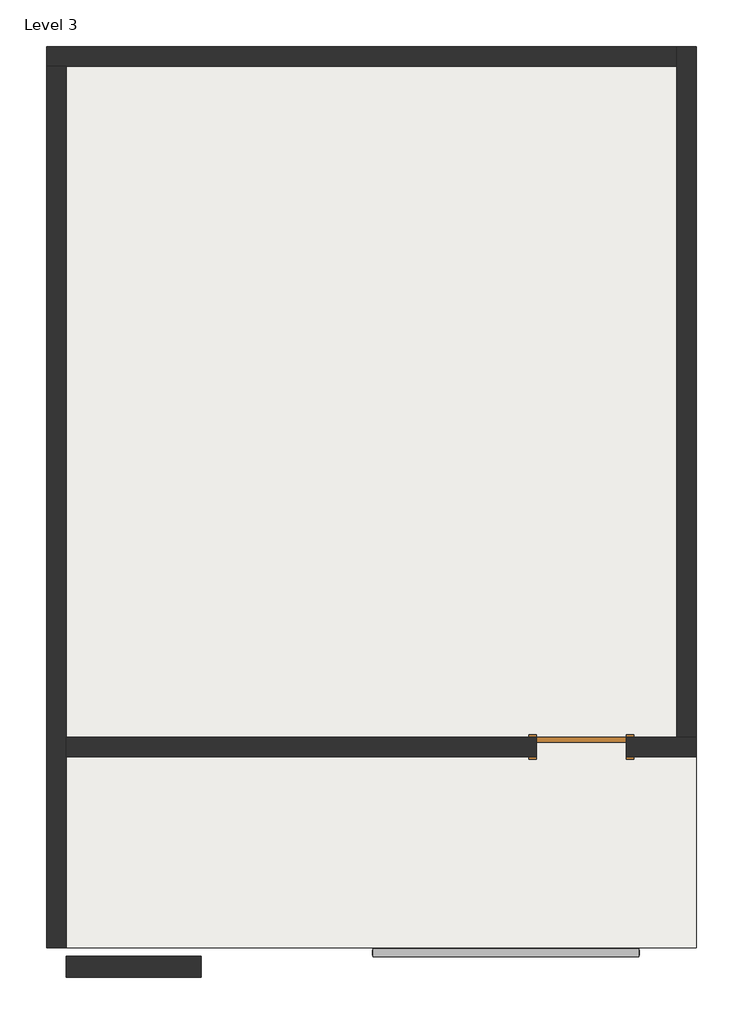
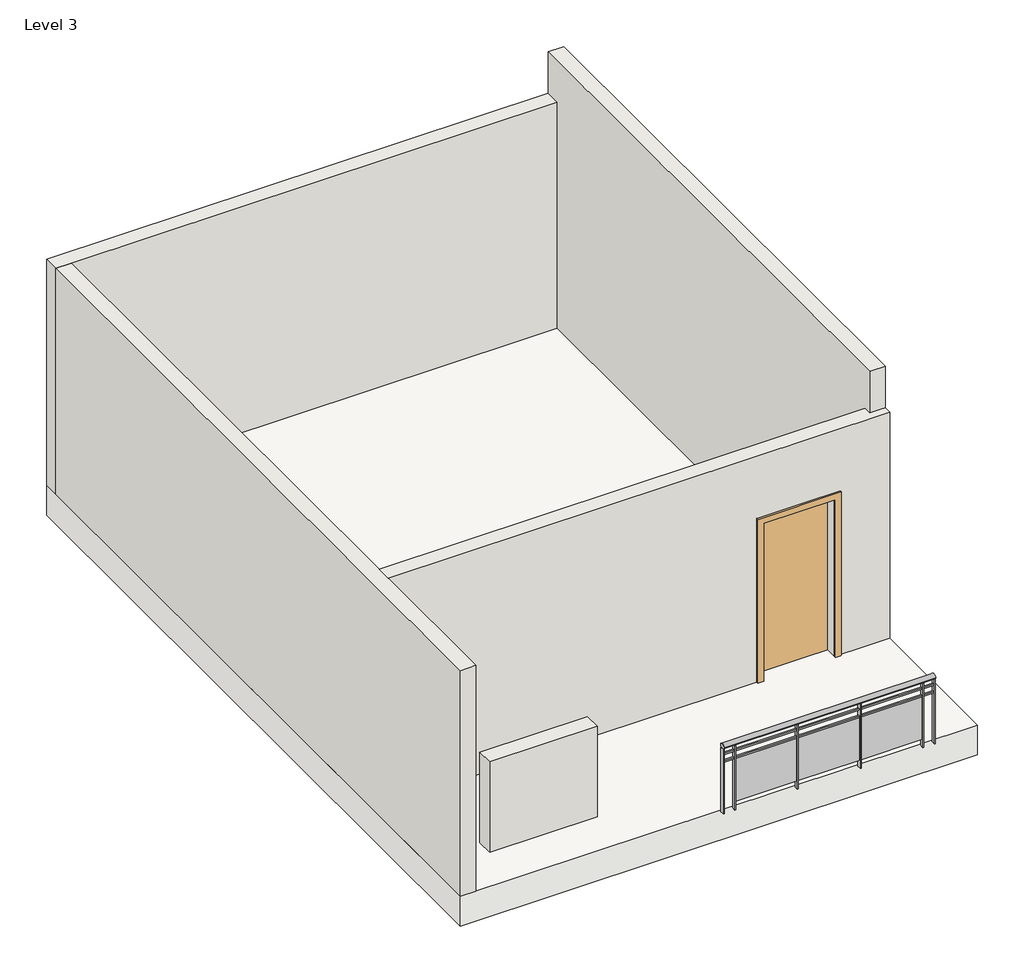
# One storey: 5 walls, 1 door, 1 railing, 1 slab.
"""IFC4 building model written with IfcOpenShell, lengths in millimetres."""

from ifc_helpers import new_model, si_unit, point, frame, origin, place, context, project, spatial, polyline, ellipse_curve, trimmed, outline, extrude, faceted_brep, transform, mapped, element, save
from ifc_brep_helpers import plane_surface, extruded_surface, advanced_brep
from components import m_single_flush_0915_x_2134mm_6a9e8738, walls_7_walls_7_d83e4491

model = new_model("IFC4")

# Units and contexts
model_context = context("Model", 3, world=origin())
ifc_project = project(units=[si_unit("LENGTHUNIT", "METRE", prefix="MILLI")], contexts=[model_context])

# Site, building, storey
site = spatial("IfcSite", under=ifc_project)
building = spatial("IfcBuilding", under=site)
storey = spatial("IfcBuildingStorey", under=building, Name="Level 3", Elevation=3048.0)

# Door
placement = place(None, origin())
m_single_flush_0915_x_2134mm_shape = m_single_flush_0915_x_2134mm_6a9e8738(model_context)
element("IfcDoor", 1, ObjectType="M_Single-Flush : 0915 x 2134mm", at=placement, inside=storey, context=model_context, shape_type="MappedRepresentation", body=[
    mapped(m_single_flush_0915_x_2134mm_shape, transform((-7079.0996792, -5453.0913939, 3048.0), x_axis=(1.0, 0.0, 0.0), y_axis=(0.0, 1.0, 0.0), z_axis=(0.0, 0.0, 1.0))),
])

# Railing
element("IfcRailing", 2, ObjectType="Glass Panel - Bottom Fill", at=placement, inside=storey, context=model_context, shape_type="SolidModel", body=[
    advanced_brep(
    [(-9197.0226654, -7500.5654668, 3948.0), (-9197.0226654, -7580.5654668, 3948.0), (-6496.1866069, -7500.5654668, 3948.0), (-6496.1866069, -7580.5654668, 3948.0)],
    [
        (0, 1, ellipse_curve(frame((-9197.0226654, -7540.5654668, 3948.0), z_axis=(-1.0, 0.0, 0.0), x_axis=(0.0, -1.0, 0.0)), 40.0, 30.0)),
        (1, 0, ellipse_curve(frame((-9197.0226654, -7540.5654668, 3948.0), z_axis=(-1.0, 0.0, 0.0), x_axis=(0.0, -1.0, 0.0)), 40.0, 30.0)),
        (2, 3, ellipse_curve(frame((-6496.1866069, -7540.5654668, 3948.0), z_axis=(1.0, 0.0, 0.0), x_axis=(0.0, -1.0, 0.0)), 40.0, 30.0)),
        (3, 2, ellipse_curve(frame((-6496.1866069, -7540.5654668, 3948.0), z_axis=(1.0, 0.0, 0.0), x_axis=(0.0, -1.0, 0.0)), 40.0, 30.0)),
        (1, 3),
        (2, 0),
    ],
    [
        plane_surface(frame((-9197.0226654, -7540.5654668, 3948.0), z_axis=(-1.0, 0.0, 0.0), x_axis=(0.0, 1.0, 0.0))),
        plane_surface(frame((-6496.1866069, -7540.5654668, 3948.0), z_axis=(1.0, 0.0, 0.0), x_axis=(0.0, 1.0, 0.0))),
        extruded_surface(trimmed(ellipse_curve(frame((-6496.1866069, -7540.5654668, 3948.0), z_axis=(-1.0, 0.0, 0.0), x_axis=(0.0, -1.0, 0.0)), 40.0, 30.0), [point((-6496.1866069, -7580.5654668, 3948.0))], [point((-6496.1866069, -7500.5654668, 3948.0))], True, "CARTESIAN"), (-2700.8360585, 0.0, 0.0), 2700.8360585),
        extruded_surface(trimmed(ellipse_curve(frame((-6496.1866069, -7540.5654668, 3948.0), z_axis=(-1.0, 0.0, 0.0), x_axis=(0.0, -1.0, 0.0)), 40.0, 30.0), [point((-6496.1866069, -7500.5654668, 3948.0))], [point((-6496.1866069, -7580.5654668, 3948.0))], True, "CARTESIAN"), (-2700.8360585, 0.0, 0.0), 2700.8360585),
    ],
    [
        (0, [[1, 2]]),
        (1, [[3, 4]]),
        (2, [[-2, 5, -3, 6]]),
        (3, [[-1, -6, -4, -5]]),
    ],
),
    extrude(outline(polyline([(-9197.0226654, -7549.9562319), (-9197.0226654, -7529.9562319), (-6496.1866069, -7529.9562319), (-6496.1866069, -7549.9562319), (-9197.0226654, -7549.9562319)])), frame((0.0, 0.0, 3828.0), z_axis=(0.0, 0.0, 1.0), x_axis=(1.0, 0.0, 0.0)), (0.0, 0.0, 1.0), 20.0),
    extrude(outline(polyline([(-9197.0226654, -7549.9562319), (-9197.0226654, -7529.9562319), (-6496.1866069, -7529.9562319), (-6496.1866069, -7549.9562319), (-9197.0226654, -7549.9562319)])), frame((0.0, 0.0, 3728.0), z_axis=(0.0, 0.0, 1.0), x_axis=(1.0, 0.0, 0.0)), (0.0, 0.0, 1.0), 20.0),
    extrude(outline(polyline([(-6652.6046361, -7514.9562319), (-6640.6046361, -7514.9562319), (-6640.6046361, -7564.9562319), (-6652.6046361, -7564.9562319), (-6652.6046361, -7514.9562319)])), frame((0.0, 0.0, 3048.0), z_axis=(0.0, 0.0, 1.0), x_axis=(1.0, 0.0, 0.0)), (0.0, 0.0, 1.0), 869.8465326),
    extrude(outline(polyline([(-7446.6046361, -7541.681042), (-6646.6046361, -7541.681042), (-6646.6046361, -7546.681042), (-7446.6046361, -7546.681042), (-7446.6046361, -7541.681042)])), frame((0.0, 0.0, 3148.0), z_axis=(0.0, 0.0, 1.0), x_axis=(1.0, 0.0, 0.0)), (0.0, 0.0, 1.0), 580.0),
    extrude(outline(polyline([(-7452.6046361, -7514.9562319), (-7440.6046361, -7514.9562319), (-7440.6046361, -7564.9562319), (-7452.6046361, -7564.9562319), (-7452.6046361, -7514.9562319)])), frame((0.0, 0.0, 3048.0), z_axis=(0.0, 0.0, 1.0), x_axis=(1.0, 0.0, 0.0)), (0.0, 0.0, 1.0), 869.8465326),
    extrude(outline(polyline([(-8246.6046361, -7541.681042), (-7446.6046361, -7541.681042), (-7446.6046361, -7546.681042), (-8246.6046361, -7546.681042), (-8246.6046361, -7541.681042)])), frame((0.0, 0.0, 3148.0), z_axis=(0.0, 0.0, 1.0), x_axis=(1.0, 0.0, 0.0)), (0.0, 0.0, 1.0), 580.0),
    extrude(outline(polyline([(-8252.6046361, -7514.9562319), (-8240.6046361, -7514.9562319), (-8240.6046361, -7564.9562319), (-8252.6046361, -7564.9562319), (-8252.6046361, -7514.9562319)])), frame((0.0, 0.0, 3048.0), z_axis=(0.0, 0.0, 1.0), x_axis=(1.0, 0.0, 0.0)), (0.0, 0.0, 1.0), 869.8465326),
    extrude(outline(polyline([(-9046.6046361, -7541.681042), (-8246.6046361, -7541.681042), (-8246.6046361, -7546.681042), (-9046.6046361, -7546.681042), (-9046.6046361, -7541.681042)])), frame((0.0, 0.0, 3148.0), z_axis=(0.0, 0.0, 1.0), x_axis=(1.0, 0.0, 0.0)), (0.0, 0.0, 1.0), 580.0),
    extrude(outline(polyline([(-9052.6046361, -7514.9562319), (-9040.6046361, -7514.9562319), (-9040.6046361, -7564.9562319), (-9052.6046361, -7564.9562319), (-9052.6046361, -7514.9562319)])), frame((0.0, 0.0, 3048.0), z_axis=(0.0, 0.0, 1.0), x_axis=(1.0, 0.0, 0.0)), (0.0, 0.0, 1.0), 869.8465326),
    extrude(outline(polyline([(-6504.1866069, -7514.9562319), (-6492.1866069, -7514.9562319), (-6492.1866069, -7564.9562319), (-6504.1866069, -7564.9562319), (-6504.1866069, -7514.9562319)])), frame((0.0, 0.0, 3048.0), z_axis=(0.0, 0.0, 1.0), x_axis=(1.0, 0.0, 0.0)), (0.0, 0.0, 1.0), 869.8465326),
    extrude(outline(polyline([(-9201.0226654, -7514.9562319), (-9189.0226654, -7514.9562319), (-9189.0226654, -7564.9562319), (-9201.0226654, -7564.9562319), (-9201.0226654, -7514.9562319)])), frame((0.0, 0.0, 3048.0), z_axis=(0.0, 0.0, 1.0), x_axis=(1.0, 0.0, 0.0)), (0.0, 0.0, 1.0), 869.8465326),
])

# Slab
element("IfcSlab", 3, ObjectType="Generic Floor - 400mm", at=placement, inside=storey, context=model_context, shape_type="SweptSolid", body=[
    extrude(outline(polyline([(-5912.2996792, 1657.3086061), (-5912.2996792, -7490.0501996), (-12513.0996792, -7490.0501996), (-12513.0996792, 1657.3086061), (-5912.2996792, 1657.3086061)])), frame((0.0, 0.0, 2648.0), z_axis=(0.0, 0.0, 1.0), x_axis=(1.0, 0.0, 0.0)), (0.0, 0.0, 1.0), 400.0),
])

# Walls
element("IfcWall", 4, ObjectType="Generic - 9\"", at=placement, inside=storey, context=model_context, shape_type="Brep", body=[
    faceted_brep([(-12513.0996792, 1457.3086061, 3048.0), (-12313.0996792, 1457.3086061, 3048.0), (-6112.2996792, 1457.3086061, 3048.0), (-6112.2996792, 1457.3086061, 6096.0), (-12313.0996792, 1457.3086061, 6096.0), (-12513.0996792, 1457.3086061, 6096.0), (-12513.0996792, 1657.3086061, 3048.0), (-12513.0996792, 1657.3086061, 6096.0), (-6112.2996792, 1657.3086061, 6096.0), (-6112.2996792, 1657.3086061, 3048.0)], [[[0, 1, 2, 3, 4, 5]], [[6, 7, 8, 9]], [[2, 1, 0, 6, 9]], [[5, 4, 3, 8, 7]], [[0, 5, 7, 6]], [[3, 2, 9, 8]]]),
])
element("IfcWall", 5, ObjectType="Generic - 9\"", at=placement, inside=storey, context=model_context, shape_type="Brep", body=[
    faceted_brep([(-12313.0996792, -7490.0501996, 3048.0), (-12313.0996792, -5553.0913939, 3048.0), (-12313.0996792, -5353.0913939, 3048.0), (-12313.0996792, 1457.3086061, 3048.0), (-12313.0996792, 1457.3086061, 6096.0), (-12313.0996792, -5353.0913939, 6096.0), (-12313.0996792, -5553.0913939, 6096.0), (-12313.0996792, -7490.0501996, 6096.0), (-12513.0996792, -7490.0501996, 3048.0), (-12513.0996792, -7490.0501996, 6096.0), (-12513.0996792, 1457.3086061, 6096.0), (-12513.0996792, 1457.3086061, 3048.0)], [[[0, 1, 2, 3, 4, 5, 6, 7]], [[8, 9, 10, 11]], [[3, 2, 1, 0, 8, 11]], [[7, 6, 5, 4, 10, 9]], [[0, 7, 9, 8]], [[4, 3, 11, 10]]]),
])
element("IfcWall", 6, ObjectType="Generic - 9\"", at=placement, inside=storey, context=model_context, shape_type="Brep", body=[
    faceted_brep([(-5912.2996792, -5353.0913939, 3048.0), (-6112.2996792, -5353.0913939, 3048.0), (-6621.5996792, -5353.0913939, 3048.0), (-6621.5996792, -5353.0913939, 5182.0), (-7536.5996792, -5353.0913939, 5182.0), (-7536.5996792, -5353.0913939, 3048.0), (-12313.0996792, -5353.0913939, 3048.0), (-12313.0996792, -5353.0913939, 6096.0), (-6112.2996792, -5353.0913939, 6096.0), (-5912.2996792, -5353.0913939, 6096.0), (-6621.5996792, -5553.0913939, 5182.0), (-6621.5996792, -5553.0913939, 3048.0), (-5912.2996792, -5553.0913939, 3048.0), (-5912.2996792, -5553.0913939, 6096.0), (-12313.0996792, -5553.0913939, 6096.0), (-12313.0996792, -5553.0913939, 3048.0), (-7536.5996792, -5553.0913939, 3048.0), (-7536.5996792, -5553.0913939, 5182.0), (-5912.2996792, -5453.0913939, 6096.0)], [[[0, 1, 2, 3, 4, 5, 6, 7, 8, 9]], [[10, 11, 12, 13, 14, 15, 16, 17]], [[16, 15, 6, 5]], [[12, 11, 2, 1, 0]], [[9, 8, 7, 14, 13, 18]], [[0, 9, 18, 13, 12]], [[3, 2, 11, 10]], [[4, 3, 10, 17]], [[5, 4, 17, 16]], [[7, 6, 15, 14]]]),
])
element("IfcWall", 7, ObjectType="Generic - 9\"", at=placement, inside=storey, context=model_context, shape_type="Brep", body=[
    faceted_brep([(-6112.2996792, 1657.3086061, 3048.0), (-6112.2996792, 1457.3086061, 3048.0), (-6112.2996792, -5353.0913939, 3048.0), (-6112.2996792, -5353.0913939, 6096.0), (-6112.2996792, -5453.0913939, 6096.0), (-6112.2996792, -5453.0913939, 6658.5115849), (-6112.2996792, 1657.3086061, 6658.5115849), (-6112.2996792, 1657.3086061, 6096.0), (-5912.2996792, 1657.3086061, 3048.0), (-5912.2996792, 1657.3086061, 6658.5115849), (-5912.2996792, -5453.0913939, 6658.5115849), (-5912.2996792, -5453.0913939, 6096.0), (-5912.2996792, -5353.0913939, 6096.0), (-5912.2996792, -5353.0913939, 3048.0)], [[[0, 1, 2, 3, 4, 5, 6, 7]], [[8, 9, 10, 11, 12, 13]], [[2, 1, 0, 8, 13]], [[6, 5, 10, 9]], [[0, 7, 6, 9, 8]], [[5, 4, 11, 10]], [[11, 4, 3, 12]], [[3, 2, 13, 12]]]),
])
walls_7_walls_7_shape = walls_7_walls_7_d83e4491(model_context)
element("IfcWall", 8, ObjectType="Walls 7 : Walls 7", at=placement, inside=storey, context=model_context, shape_type="MappedRepresentation", body=[
    mapped(walls_7_walls_7_shape, transform((0.0, 0.0, 0.0), x_axis=(1.0, 0.0, 0.0), y_axis=(0.0, 1.0, 0.0), z_axis=(0.0, 0.0, 1.0))),
])

save(model, "model.ifc")

# Revit data of these elements
# Type "M_Single-Flush : 0915 x 2134mm"
#   Type Mark = "15"
#   Thickness = 51 mm
#   Height = 2134 mm
#   Trim Projection Ext = 25 mm
#   Trim Projection Int = 25 mm
#   Trim Width = 76 mm
#   Width = 915 mm
#   Door Material = Door - Panel
#   Frame Material = Door - Frame
#   Function = (empty or 0)
#   Wall Closure = (empty or 0)
# Type "Glass Panel - Bottom Fill"
#   built-in parameter 1008612 = 0.019685 (stored number, unit not read)
#   built-in parameter 1008611 = 0.019685 (stored number, unit not read)
#   built-in parameter 1008609 = 0.902231 (stored number, unit not read)
#   built-in parameter 1008604 = 0.19685 (stored number, unit not read)
#   built-in parameter 1008603 = 0.164042 (stored number, unit not read)
#   Railing Height = 900 mm
#   built-in parameter 1008630 = 2
#   built-in parameter 1008610 = 2
# Type "Generic Floor - 400mm"
#   Function = 0
#   Layers, outside or top first: 400 mm no material (function 1)
# Type "Generic - 9\""
#   Layers, outside or top first: 200 mm no material (function 1)
# Element 1 (IfcDoor, "M_Single-Flush : 0915 x 2134mm")
#   Phase Created = New Construction
#   Materials on its faces: "Door - Frame", "Door - Panel"
# Element 2 (IfcRailing, "Glass Panel - Bottom Fill")
#   Phase Created = New Construction
#   Materials on its faces: "Metal - Stainless Steel,Polished", "Glass"
# Element 3 (IfcSlab, "Generic Floor - 400mm")
#   Height Offset From Level = 0 mm
#   Phase Created = New Construction
#   Materials on its faces: "Default Roof"
# Elements 4, 5, 6 (IfcWall, "Generic - 9\"")
#   Top Offset = 0 mm
#   Base Offset = 0 mm
#   Unconnected Height = 3048 mm
#   wall height = 3048 mm
#   Phase Created = New Construction
#   Base Constraint = Level 3
#   Materials on its faces: "Default Wall"
# Element 7 (IfcWall, "Generic - 9\"")
#   Top Offset = 0 mm
#   Base Offset = 0 mm
#   Unconnected Height = 3610.512 mm
#   wall height = 3610.512 mm
#   Phase Created = New Construction
#   Base Constraint = Level 3
#   Materials on its faces: "Default Wall"
# Element 8 (IfcWall, "Walls 7 : Walls 7")
#   Phase Created = New Construction
#   Materials on its faces: "Default Wall"
# Materials
#   "Door - Panel": class "Wood", colour RGB 114 82 51, transparency 0
#   "Door - Frame": colour RGB 153 76 43, transparency 0
#   "Metal - Stainless Steel,Polished": class "Metal", colour RGB 189 187 185, transparency 0, Cost = 0
#   "Glass": class "Glass", colour RGB 218 227 224, transparency 0.85, Description = "Soda Lime Glass", Cost = 0
#   "Default Roof": colour RGB 80 80 80, transparency 0
#   "Default Wall": colour RGB 80 80 80, transparency 0
